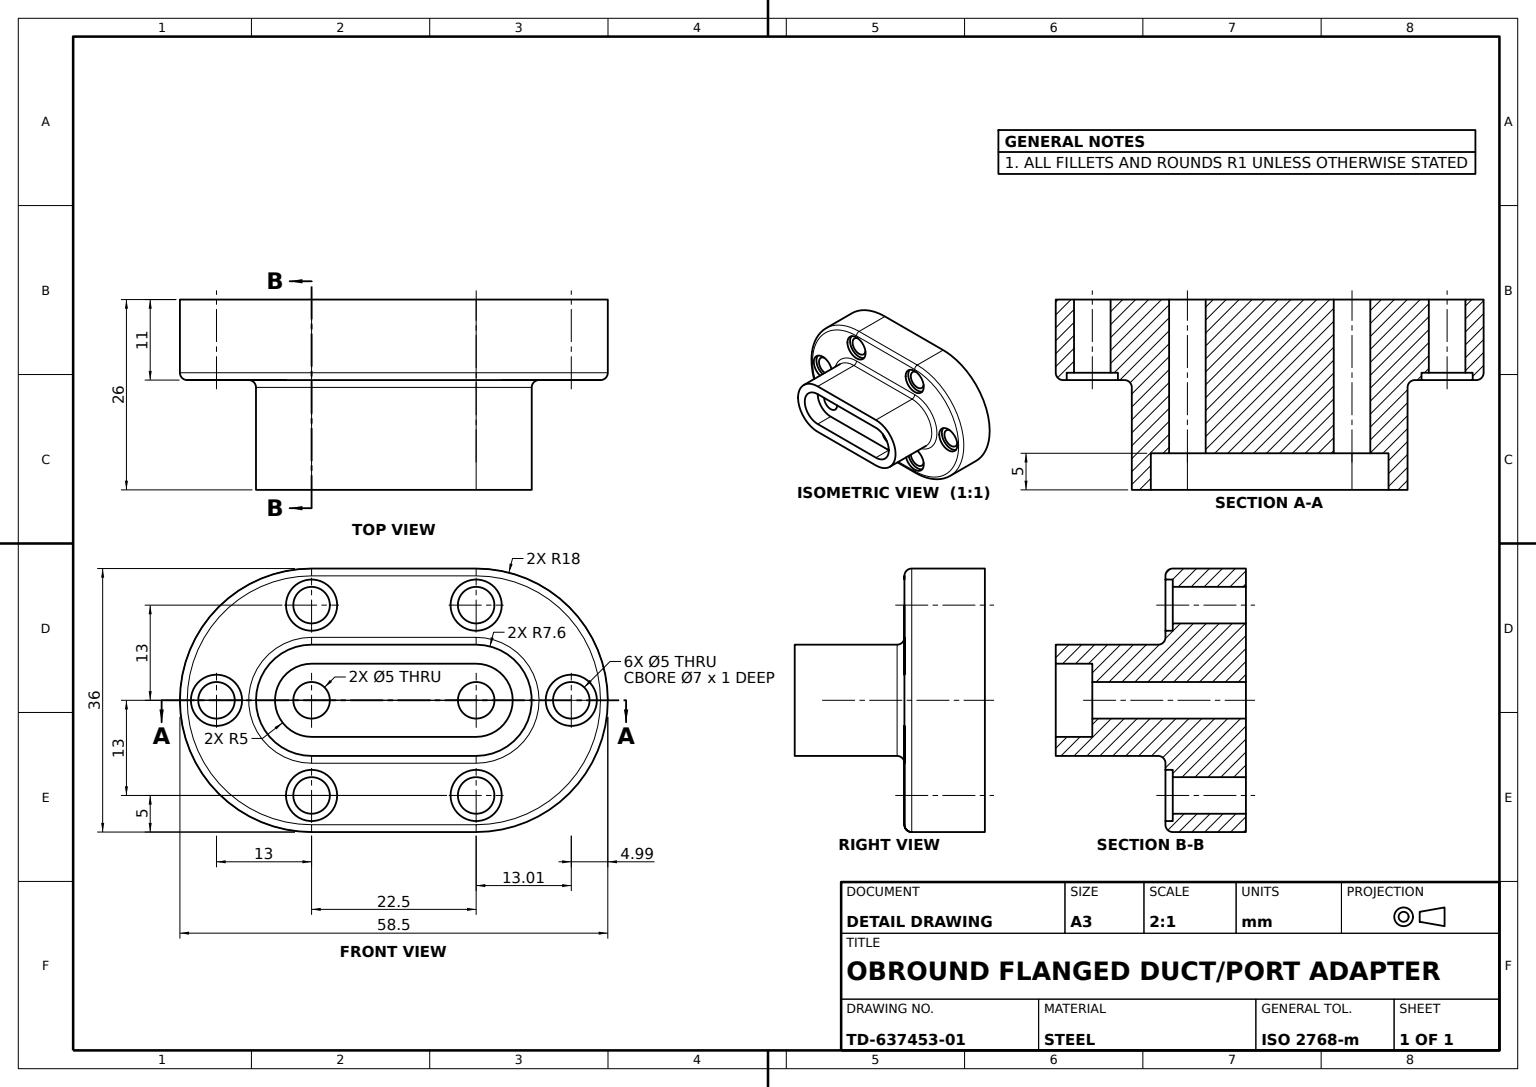
from build123d import *

# Parameters (mm, degrees)
BASE_FLANGE_DEPTH          = 11
OBROUND_BOSS_DEPTH         = 15
BOSS_POCKET_DEPTH          = 5
MOUNTING_HOLES_A_PROFILE_R = 2.5
MOUNTING_HOLES_A_DEPTH     = 47.789421881
SPOT_FACES_A_PROFILE_R     = 3.5
SPOT_FACES_A_DEPTH         = 1
CENTRE_HOLES_PROFILE_R     = 2.5
CENTRE_HOLES_DEPTH         = 50.043348173
BOSS_ROOT_FILLET_R1_R      = 1
MOUNTING_HOLES_B_PROFILE_R = 2.5
MOUNTING_HOLES_B_DEPTH     = 47.789421881
SPOT_FACES_B_PROFILE_R     = 3.5
SPOT_FACES_B_DEPTH         = 1


with BuildPart() as part:
    # Flange Profile → Base Flange (new body)
    with BuildSketch(Plane.XY):
        with BuildLine():
            Line((0, 18), (22.5, 18))
            ThreePointArc((22.5, 18), (40.5, 0), (22.5, -18))
            Line((22.5, -18), (0, -18))
            ThreePointArc((0, -18), (-18, 0), (0, 18))
        make_face()
    extrude(amount=BASE_FLANGE_DEPTH)

    # Boss Profile → Obround Boss (add)
    with BuildSketch(Plane.XY.offset(11)):
        with BuildLine():
            Line((0, 7.6), (22.5, 7.6))
            ThreePointArc((22.5, 7.6), (30.1, 0), (22.5, -7.6))
            Line((22.5, -7.6), (0, -7.6))
            ThreePointArc((0, -7.6), (-7.6, 0), (0, 7.6))
        make_face()
    extrude(amount=OBROUND_BOSS_DEPTH)

    # Boss Pocket Profile → Boss Pocket (cut)
    with BuildSketch(Plane.XY.offset(26)):
        with BuildLine():
            Line((0, 5), (22.5, 5))
            ThreePointArc((22.5, 5), (27.5, 0), (22.5, -5))
            Line((22.5, -5), (0, -5))
            ThreePointArc((0, -5), (-5, 0), (0, 5))
        make_face()
    extrude(amount=-BOSS_POCKET_DEPTH, mode=Mode.SUBTRACT)

    # Mounting Holes A Profile → Mounting Holes A (cut, through all)
    with BuildSketch(Plane.XY.offset(11)):
        with Locations((0, 13)):
            Circle(MOUNTING_HOLES_A_PROFILE_R)
        with Locations((22.5, 13)):
            Circle(MOUNTING_HOLES_A_PROFILE_R)
        with Locations((0, -13)):
            Circle(MOUNTING_HOLES_A_PROFILE_R)
        with Locations((22.5, -13)):
            Circle(MOUNTING_HOLES_A_PROFILE_R)
    extrude(amount=-MOUNTING_HOLES_A_DEPTH, mode=Mode.SUBTRACT)

    # Spot Faces A Profile → Spot Faces A (cut)
    with BuildSketch(Plane.XY.offset(11)):
        with Locations((0, 13)):
            Circle(SPOT_FACES_A_PROFILE_R)
        with Locations((22.5, 13)):
            Circle(SPOT_FACES_A_PROFILE_R)
        with Locations((22.5, -13)):
            Circle(SPOT_FACES_A_PROFILE_R)
        with Locations((0, -13)):
            Circle(SPOT_FACES_A_PROFILE_R)
    extrude(amount=-SPOT_FACES_A_DEPTH, mode=Mode.SUBTRACT)

    # Centre Holes Profile → Centre Holes (cut, through all)
    with BuildSketch(Plane.XY.offset(21)):
        Circle(CENTRE_HOLES_PROFILE_R)
        with Locations((22.50803184, 0)):
            Circle(CENTRE_HOLES_PROFILE_R)
    extrude(amount=-CENTRE_HOLES_DEPTH, mode=Mode.SUBTRACT)

    # Boss Root Fillet R1
    boss_root_fillet_r1_edges = [part.edges().sort_by_distance(p)[0] for p in [
        (40.5, 0, 11),
        (-7.6, 0, 11),
        (11.25, -7.6, 11),
        (11.25, 18, 11),
        (30.1, 0, 11),
        (11.25, 7.6, 11),
        (-18, 0, 11),
        (11.25, -18, 11),
    ]]
    fillet(boss_root_fillet_r1_edges, radius=BOSS_ROOT_FILLET_R1_R)

    # Mounting Holes B Profile → Mounting Holes B (cut, through all)
    with BuildSketch(Plane.XY.offset(11)):
        with Locations((-13, 0)):
            Circle(MOUNTING_HOLES_B_PROFILE_R)
        with Locations((35.50803184, 0)):
            Circle(MOUNTING_HOLES_B_PROFILE_R)
    extrude(amount=-MOUNTING_HOLES_B_DEPTH, mode=Mode.SUBTRACT)

    # Spot Faces B Profile → Spot Faces B (cut)
    with BuildSketch(Plane.XY.offset(11)):
        with Locations((-13, 0)):
            Circle(SPOT_FACES_B_PROFILE_R)
        with Locations((35.50803184, 0)):
            Circle(SPOT_FACES_B_PROFILE_R)
    extrude(amount=-SPOT_FACES_B_DEPTH, mode=Mode.SUBTRACT)


solid = part.part
